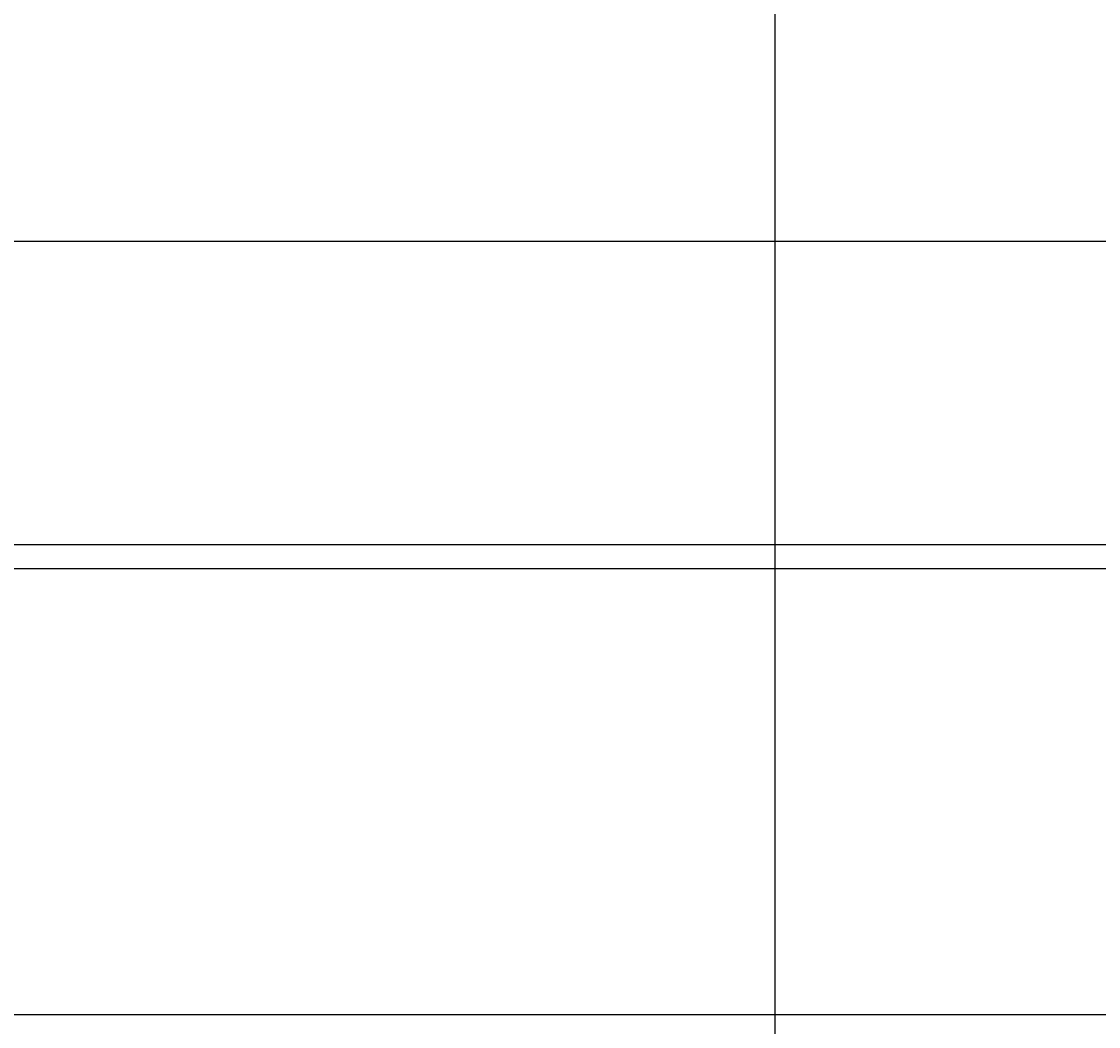
# Model space of a CAD drawing. Units: inches. Extents: x 35362 to 73946, y 43607 to 67532.
# Tile 133 of 134: x 66704 to 67594, y 45460 to 46290. Entities that reach past the tile are written whole.
import ezdxf

# ---------------------------------------------------------------- set-up
doc = ezdxf.new("R2010")
doc.units = ezdxf.units.IN
doc.header["$MEASUREMENT"] = 0
doc.layers.add('A-ANNO-DIMS', color=2, linetype='Continuous', lineweight=18)
doc.styles.get("Standard").update_dxf_attribs({"font": 'arial.ttf'})
doc.dimstyles.get("Standard").update_dxf_attribs({"dimtxt": 0.18, "dimasz": 0.18, "dimexe": 0.18, "dimexo": 0.0625, "dimgap": 0.09, "dimtad": 0, "dimtih": 1, "dimtoh": 1, "dimdec": 4, "dimzin": 0, "dimdsep": 46, "dimtxsty": 'Standard', "dimcen": 0.09, "dimadec": 0, "dimazin": 0, "dimtfac": 1, "dimtdec": 4, "dimtofl": 0, "dimtmove": 0, "dimatfit": 3, "dimfxl": 1, "dimtolj": 1, "dimtzin": 0, "dimarcsym": 0})

# ---------------------------------------------------------------- blocks, each defined once
blk = doc.blocks.new('*D5')
at = {"layer": 'A-ANNO-DIMS', "color": 0, "lineweight": -2, "transparency": 16777216}
for p, q in [((37121.949085, 46919.318283), (37121.949085, 43606.678996)), ((69871.496302, 45449.831951), (69871.496302, 43606.678996)), ((37122.129085, 43606.858996), (53496.2943647142, 43606.858996)), ((69871.316302, 43606.858996), (53497.15102228581, 43606.858996))]:
    blk.add_line(p, q, dxfattribs=at)
at = {"layer": 'A-ANNO-DIMS', "color": 0, "transparency": 16777216}
for points in [[(37122.129085, 43606.888996), (37122.129085, 43606.828996), (37121.949085, 43606.858996)], [(69871.316302, 43606.888996), (69871.316302, 43606.828996), (69871.496302, 43606.858996)]]:
    blk.add_solid(points, dxfattribs=at)
at = {"layer": 'Defpoints', "color": 0, "transparency": 16777216}
for p in [(37121.949085, 46919.380783), (69871.496302, 45449.894451), (69871.496302, 43606.858996)]:
    blk.add_point(p, dxfattribs=at)
at = {"layer": 'A-ANNO-DIMS', "color": 0, "transparency": 16777216, "insert": (53496.7226935, 43606.858996), "char_height": 0.18, "attachment_point": 5}
blk.add_mtext('\\A1;32750', dxfattribs=at)
blk = doc.blocks.new('*D65')
at = {"layer": 'A-ANNO-DIMS', "color": 0, "lineweight": -2, "transparency": 16777216}
for p, q in [((65336.01600799999, 61293.223552), (65336.01600799999, 43606.678996)), ((67326.639741, 61293.223552), (67326.639741, 43606.678996)), ((65336.19600799999, 43606.858996), (66330.87277900206, 43606.858996)), ((67326.45974100001, 43606.858996), (66331.78296999796, 43606.858996))]:
    blk.add_line(p, q, dxfattribs=at)
at = {"layer": 'A-ANNO-DIMS', "color": 0, "transparency": 16777216}
for points in [[(65336.19600799999, 43606.888996), (65336.19600799999, 43606.828996), (65336.01600799999, 43606.858996)], [(67326.45974100001, 43606.888996), (67326.45974100001, 43606.828996), (67326.639741, 43606.858996)]]:
    blk.add_solid(points, dxfattribs=at)
at = {"layer": 'Defpoints', "color": 0, "transparency": 16777216}
for p in [(65336.01600799999, 61293.286052), (67326.639741, 61293.286052), (67326.639741, 43606.858996)]:
    blk.add_point(p, dxfattribs=at)
at = {"layer": 'A-ANNO-DIMS', "color": 0, "transparency": 16777216, "insert": (66331.32787450001, 43606.858996), "char_height": 0.18, "attachment_point": 5}
blk.add_mtext('\\A1;1990.6', dxfattribs=at)
blk = doc.blocks.new('*D68')
at = {"layer": 'A-ANNO-DIMS', "color": 0, "lineweight": -2, "transparency": 16777216}
for p, q in [((68320.870762, 54372.885224), (68320.870762, 43606.678996)), ((61240.907336, 53351.466162), (61240.907336, 43606.678996)), ((61241.08733599999, 43606.858996), (64780.42646373397, 43606.858996)), ((68320.69076200001, 43606.858996), (64781.35163426603, 43606.858996))]:
    blk.add_line(p, q, dxfattribs=at)
at = {"layer": 'A-ANNO-DIMS', "color": 0, "transparency": 16777216}
for points in [[(61241.08733599999, 43606.888996), (61241.08733599999, 43606.828996), (61240.907336, 43606.858996)], [(68320.69076200001, 43606.888996), (68320.69076200001, 43606.828996), (68320.870762, 43606.858996)]]:
    blk.add_solid(points, dxfattribs=at)
at = {"layer": 'Defpoints', "color": 0, "transparency": 16777216}
for p in [(68320.870762, 54372.947724), (61240.907336, 53351.52866199999), (68320.870762, 43606.858996)]:
    blk.add_point(p, dxfattribs=at)
at = {"layer": 'A-ANNO-DIMS', "color": 0, "transparency": 16777216, "insert": (64780.889049, 43606.858996), "char_height": 0.18, "attachment_point": 5}
blk.add_mtext('\\A1;7080.0', dxfattribs=at)
blk = doc.blocks.new('*D74')
at = {"layer": 'A-ANNO-DIMS', "color": 0, "lineweight": -2, "transparency": 16777216}
for p, q in [((55181.69646300003, 46108.87757800001), (73945.82566600003, 46108.87757800001)), ((73945.64566600005, 46108.69757800001), (73945.64566600005, 45983.7251866378)), ((73945.64566600005, 45858.38898900001), (73945.64566600005, 45983.36138036223)), ((55181.69646300003, 45858.20898900001), (73945.82566600003, 45858.20898900001))]:
    blk.add_line(p, q, dxfattribs=at)
at = {"layer": 'A-ANNO-DIMS', "color": 0, "transparency": 16777216}
for points in [[(73945.61566600006, 46108.69757800001), (73945.67566600005, 46108.69757800001), (73945.64566600005, 46108.87757800001)], [(73945.61566600006, 45858.38898900001), (73945.67566600005, 45858.38898900001), (73945.64566600005, 45858.20898900001)]]:
    blk.add_solid(points, dxfattribs=at)
at = {"layer": 'Defpoints', "color": 0, "transparency": 16777216}
for p in [(55181.63396300002, 46108.87757800001), (55181.63396300002, 45858.20898900001), (73945.64566600005, 45858.20898900001)]:
    blk.add_point(p, dxfattribs=at)
at = {"layer": 'A-ANNO-DIMS', "color": 0, "transparency": 16777216, "insert": (73945.64566600005, 45983.54328349999), "char_height": 0.18, "attachment_point": 5}
blk.add_mtext('\\A1;250.67', dxfattribs=at)
blk = doc.blocks.new('*D75')
at = {"layer": 'A-ANNO-DIMS', "color": 0, "lineweight": -2, "transparency": 16777216}
for p, q in [((55181.69646300003, 45838.20898900001), (73945.82566600003, 45838.20898900001)), ((73945.64566600005, 45838.02898900001), (73945.64566600005, 45654.23368452933)), ((73945.64566600005, 45470.07445100001), (73945.64566600005, 45653.86975547068)), ((55181.69646300003, 45469.89445100001), (73945.82566600003, 45469.89445100001))]:
    blk.add_line(p, q, dxfattribs=at)
at = {"layer": 'A-ANNO-DIMS', "color": 0, "transparency": 16777216}
for points in [[(73945.61566600006, 45838.02898900001), (73945.67566600005, 45838.02898900001), (73945.64566600005, 45838.20898900001)], [(73945.61566600006, 45470.07445100001), (73945.67566600005, 45470.07445100001), (73945.64566600005, 45469.89445100001)]]:
    blk.add_solid(points, dxfattribs=at)
at = {"layer": 'Defpoints', "color": 0, "transparency": 16777216}
for p in [(55181.63396300002, 45838.20898900001), (55181.63396300002, 45469.89445100001), (73945.64566600005, 45469.89445100001)]:
    blk.add_point(p, dxfattribs=at)
at = {"layer": 'A-ANNO-DIMS', "color": 0, "transparency": 16777216, "insert": (73945.64566600005, 45654.05171999998), "char_height": 0.18, "attachment_point": 5}
blk.add_mtext('\\A1;368.3', dxfattribs=at)

msp = doc.modelspace()

# ---------------------------------------------------------------- dimensions: what is measured, and where the dimension line sits
at = {"layer": 'A-ANNO-DIMS'}
for base, p1, p2, override, picture, middle in [((67326.639741, 43606.858996), (65336.01600799999, 61293.286052), (67326.639741, 61293.286052), {"dimdec": 1, "dimlfac": 1, "dimrnd": 0, "dimzin": 0, "dimdsep": 46, "dimlunit": 2}, '*D65', (66331.32787450001, 43606.858996)), ((68320.870762, 43606.858996), (61240.907336, 53351.52866199999), (68320.870762, 54372.947724), {"dimdec": 1, "dimlfac": 1, "dimrnd": 0, "dimzin": 0, "dimdsep": 46, "dimlunit": 2}, '*D68', (64780.889049, 43606.858996)), ((69871.496302, 43606.858996), (37121.949085, 46919.380783), (69871.496302, 45449.894451), {"dimdec": 0, "dimlfac": 1, "dimrnd": 0, "dimzin": 0, "dimdsep": 46, "dimlunit": 2}, '*D5', (53496.7226935, 43606.858996))]:
    dim = msp.add_linear_dim(base=base, p1=p1, p2=p2, dimstyle='Standard', override=override, dxfattribs=at)
    dim.commit()
    dim.dimension.update_dxf_attribs({"geometry": picture, "text_midpoint": middle})
for base, p1, p2, override, picture, middle in [((73945.64566600005, 45858.20898900001), (55181.633963, 46108.877578), (55181.633963, 45858.20898899999), {"dimdec": 2, "dimlfac": 1, "dimrnd": 0, "dimzin": 0, "dimdsep": 46, "dimlunit": 2}, '*D74', (73945.64566600005, 45983.54328349999)), ((73945.64566600005, 45469.89445100001), (55181.633963, 45838.20898899999), (55181.633963, 45469.894451), {"dimdec": 1, "dimlfac": 1, "dimrnd": 0, "dimzin": 0, "dimdsep": 46, "dimlunit": 2}, '*D75', (73945.64566600005, 45654.05171999998))]:
    dim = msp.add_linear_dim(base=base, p1=p1, p2=p2, angle=90, dimstyle='Standard', override=override, dxfattribs=at)
    dim.commit()
    dim.dimension.update_dxf_attribs({"geometry": picture, "text_midpoint": middle})

doc.saveas('drawing.dxf')
